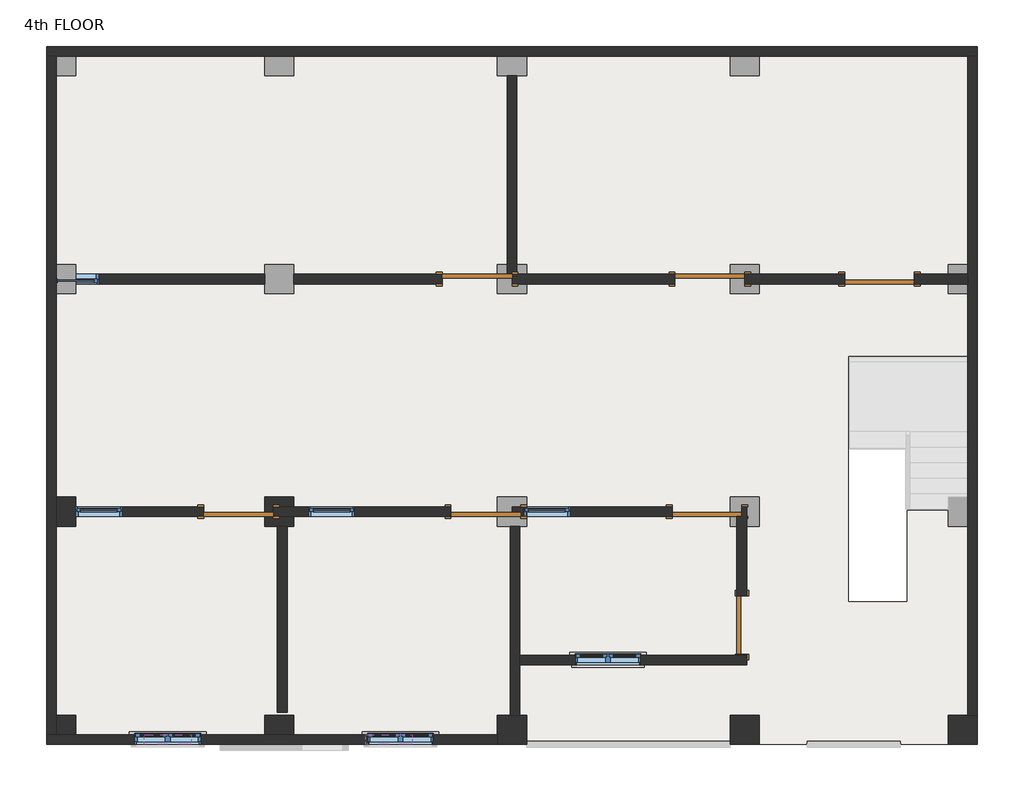
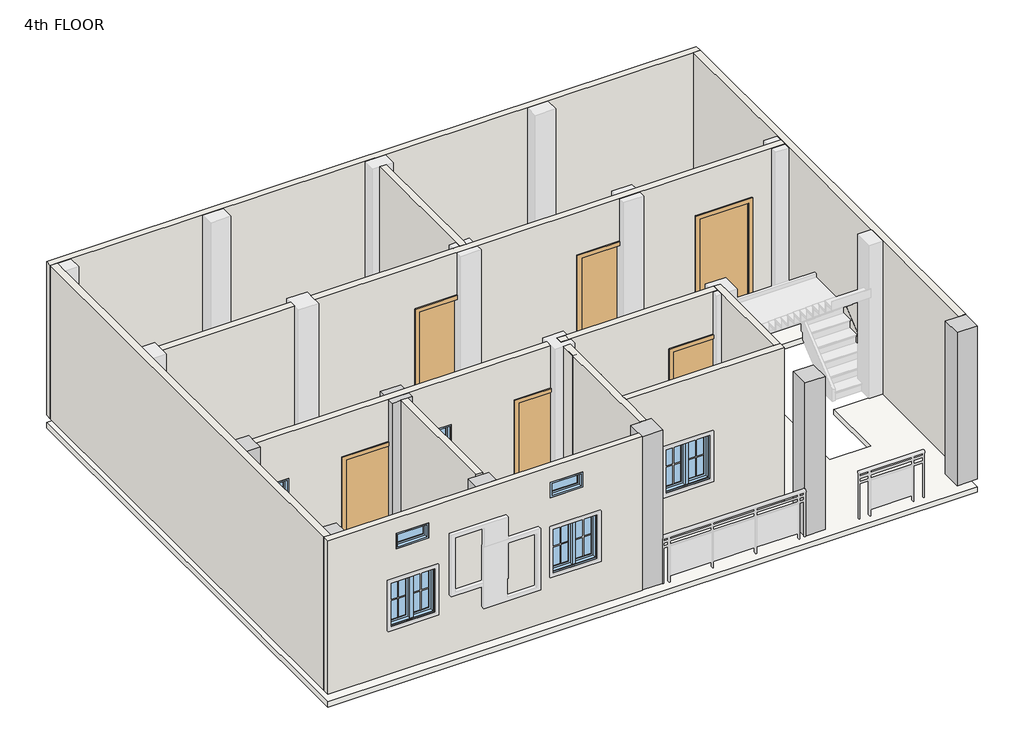
# One storey, part 1 of 2: 15 walls, 9 windows, 7 columns, 7 doors, 1 slab.
"""IFC4 building model written with IfcOpenShell, lengths in millimetres."""

from ifc_helpers import new_model, si_unit, frame, origin, place, context, project, spatial, polyline, outline, extrude, faceted_brep, transform, mapped, element, save
from components import door_e00f436c, door_a1797ceb, window_4c2727af, window_0bf3737e, window_78893e6c, window_0d9958e7

model = new_model("IFC4")

# Units and contexts
model_context = context("Model", 3, world=origin())
ifc_project = project(units=[si_unit("LENGTHUNIT", "METRE", prefix="MILLI")], contexts=[model_context])

# Site, building, storey
site = spatial("IfcSite", under=ifc_project)
building = spatial("IfcBuilding", under=site)
storey = spatial("IfcBuildingStorey", under=building, Name="4th FLOOR", Elevation=12039.6)

# Columns
placement = place(None, origin())
element("IfcColumn", 1, ObjectType="column family : column family", at=placement, inside=storey, context=model_context, shape_type="Brep", body=[
    faceted_brep([(-12576.097125, 2486.2065522, 12044.6), (-12957.097125, 2486.2065522, 12044.6), (-12957.097125, 2867.2065522, 12044.6), (-12576.097125, 2867.2065522, 12044.6), (-12576.097125, 2740.2065522, 12044.6), (-12842.797125, 2740.2065522, 12044.6), (-12842.797125, 2613.2065522, 12044.6), (-12576.097125, 2613.2065522, 12044.6), (-12576.097125, 2486.2065522, 15082.6), (-12576.097125, 2613.2065522, 15082.6), (-12957.097125, 2486.2065522, 15082.6), (-12957.097125, 2613.2065522, 15082.6), (-12957.097125, 2613.2065522, 14173.2), (-12957.097125, 2740.2065522, 14173.2), (-12957.097125, 2740.2065522, 15082.6), (-12957.097125, 2867.2065522, 15082.6), (-12576.097125, 2867.2065522, 15082.6), (-12842.797125, 2613.2065522, 14173.2), (-12842.797125, 2740.2065522, 14173.2), (-12576.097125, 2740.2065522, 15082.6)], [[[0, 1, 2, 3, 4, 5, 6, 7]], [[8, 0, 7, 9]], [[1, 0, 8, 10]], [[2, 1, 10, 11, 12, 13, 14, 15]], [[3, 2, 15, 16]], [[10, 8, 9, 11]], [[6, 17, 12, 11, 9, 7]], [[13, 18, 5, 4, 19, 14]], [[3, 16, 19, 4]], [[16, 15, 14, 19]], [[17, 18, 13, 12]], [[18, 17, 6, 5]]]),
])
element("IfcColumn", 2, ObjectType="column family : column family", at=placement, inside=storey, context=model_context, shape_type="SweptSolid", body=[
    extrude(outline(polyline([(-15433.597125, 2867.2065522), (-15433.597125, 2486.2065522), (-15687.597125, 2486.2065522), (-15687.597125, 2867.2065522), (-15433.597125, 2867.2065522)])), frame((0.0, 0.0, 12044.6), z_axis=(0.0, 0.0, 1.0), x_axis=(1.0, 0.0, 0.0)), (0.0, 0.0, 1.0), 3038.0),
])
element("IfcColumn", 3, ObjectType="column family : column family", at=placement, inside=storey, context=model_context, shape_type="SweptSolid", body=[
    extrude(outline(polyline([(-15433.597125, 9.7065522), (-15433.597125, -244.2934478), (-15687.597125, -244.2934478), (-15687.597125, 9.7065522), (-15433.597125, 9.7065522)])), frame((0.0, 0.0, 12044.6), z_axis=(0.0, 0.0, 1.0), x_axis=(1.0, 0.0, 0.0)), (0.0, 0.0, 1.0), 3038.0),
])
element("IfcColumn", 4, ObjectType="column family : column family", at=placement, inside=storey, context=model_context, shape_type="SweptSolid", body=[
    extrude(outline(polyline([(-3622.597125, 9.7065522), (-3622.597125, -371.2934478), (-4003.597125, -371.2934478), (-4003.597125, 9.7065522), (-3622.597125, 9.7065522)])), frame((0.0, 0.0, 12044.6), z_axis=(0.0, 0.0, 1.0), x_axis=(1.0, 0.0, 0.0)), (0.0, 0.0, 1.0), 3038.0),
])
element("IfcColumn", 5, ObjectType="column family : column family", at=placement, inside=storey, context=model_context, shape_type="SweptSolid", body=[
    extrude(outline(polyline([(-6480.097125, 9.7065522), (-6480.097125, -371.2934478), (-6861.097125, -371.2934478), (-6861.097125, 9.7065522), (-6480.097125, 9.7065522)])), frame((0.0, 0.0, 12044.6), z_axis=(0.0, 0.0, 1.0), x_axis=(1.0, 0.0, 0.0)), (0.0, 0.0, 1.0), 3038.0),
])
element("IfcColumn", 6, ObjectType="column family : column family", at=placement, inside=storey, context=model_context, shape_type="SweptSolid", body=[
    extrude(outline(polyline([(-9528.097125, 9.7065522), (-9528.097125, -371.2934478), (-9909.097125, -371.2934478), (-9909.097125, 9.7065522), (-9528.097125, 9.7065522)])), frame((0.0, 0.0, 12044.6), z_axis=(0.0, 0.0, 1.0), x_axis=(1.0, 0.0, 0.0)), (0.0, 0.0, 1.0), 3038.0),
])
element("IfcColumn", 7, ObjectType="column family : column family", at=placement, inside=storey, context=model_context, shape_type="SweptSolid", body=[
    extrude(outline(polyline([(-12957.097125, 9.7065522), (-12576.097125, 9.7065522), (-12576.097125, -244.2934478), (-12957.097125, -244.2934478), (-12957.097125, 9.7065522)])), frame((0.0, 0.0, 12044.6), z_axis=(0.0, 0.0, 1.0), x_axis=(1.0, 0.0, 0.0)), (0.0, 0.0, 1.0), 3038.0),
])

# Doors
door_shape = door_e00f436c(model_context)
element("IfcDoor", 8, ObjectType="Single-Flush : 30\" x 80\"", at=placement, inside=storey, context=model_context, shape_type="MappedRepresentation", body=[
    mapped(door_shape, transform((-6708.697125, 1190.8065522, 12039.6), x_axis=(0.0, -1.0, 0.0), y_axis=(1.0, 0.0, 0.0), z_axis=(0.0, 0.0, 1.0))),
])
door_2_shape = door_a1797ceb(model_context)
element("IfcDoor", 9, ObjectType="Single-Flush : 36\" x 84\"", at=placement, inside=storey, context=model_context, shape_type="MappedRepresentation", body=[
    mapped(door_2_shape, transform((-10175.797125, 5724.7065522, 12039.6), x_axis=(1.0, 0.0, 0.0), y_axis=(0.0, 1.0, 0.0), z_axis=(0.0, 0.0, 1.0))),
])
element("IfcDoor", 10, ObjectType="Single-Flush : 36\" x 84\"", at=placement, inside=storey, context=model_context, shape_type="MappedRepresentation", body=[
    mapped(door_2_shape, transform((-10061.497125, 2676.7065522, 12039.6), x_axis=(-1.0, 0.0, 0.0), y_axis=(0.0, -1.0, 0.0), z_axis=(0.0, 0.0, 1.0))),
])
element("IfcDoor", 11, ObjectType="Single-Flush : 36\" x 84\"", at=placement, inside=storey, context=model_context, shape_type="MappedRepresentation", body=[
    mapped(door_2_shape, transform((-13299.997125, 2676.7065522, 12039.6), x_axis=(-1.0, 0.0, 0.0), y_axis=(0.0, -1.0, 0.0), z_axis=(0.0, 0.0, 1.0))),
])
element("IfcDoor", 12, ObjectType="Single-Flush : 36\" x 84\"", at=placement, inside=storey, context=model_context, shape_type="MappedRepresentation", body=[
    mapped(door_2_shape, transform((-7127.797125, 5724.7065522, 12039.6), x_axis=(1.0, 0.0, 0.0), y_axis=(0.0, 1.0, 0.0), z_axis=(0.0, 0.0, 1.0))),
])
element("IfcDoor", 13, ObjectType="Single-Flush : 36\" x 84\"", at=placement, inside=storey, context=model_context, shape_type="MappedRepresentation", body=[
    mapped(door_2_shape, transform((-7165.897125, 2676.7065522, 12039.6), x_axis=(-1.0, 0.0, 0.0), y_axis=(0.0, -1.0, 0.0), z_axis=(0.0, 0.0, 1.0))),
])
element("IfcDoor", 14, ObjectType="Single-Flush : 36\" x 84\"", at=placement, inside=storey, context=model_context, shape_type="MappedRepresentation", body=[
    mapped(door_2_shape, transform((-4905.297125, 5724.7065522, 12039.6), x_axis=(-1.0, 0.0, 0.0), y_axis=(0.0, -1.0, 0.0), z_axis=(0.0, 0.0, 1.0))),
])

# Slab
element("IfcSlab", 15, ObjectType="Generic - 4\"", at=placement, inside=storey, context=model_context, shape_type="SweptSolid", body=[
    extrude(outline(polyline([(-3622.597125, 8772.7065522), (-3622.597125, -371.2934478), (-15814.597125, -371.2934478), (-15814.597125, 8772.7065522), (-3622.597125, 8772.7065522)]), holes=[polyline([(-3734.357125, 4711.0719226), (-5310.2646464, 4711.0719226), (-5310.2646464, 1502.3126957), (-4547.7736682, 1502.3126957), (-4547.7736682, 2699.911213), (-3734.357125, 2699.911213), (-3734.357125, 4711.0719226)])]), frame((0.0, 0.0, 11785.6), z_axis=(0.0, 0.0, 1.0), x_axis=(1.0, 0.0, 0.0)), (0.0, 0.0, 1.0), 101.6),
])

# Walls
element("IfcWall", 16, ObjectType="Generic - 5\"", at=placement, inside=storey, context=model_context, shape_type="Brep", body=[
    faceted_brep([(-15814.597125, 8645.7065522, 12039.6), (-15687.597125, 8645.7065522, 12039.6), (-3749.597125, 8645.7065522, 12039.6), (-3622.597125, 8645.7065522, 12039.6), (-3622.597125, 8645.7065522, 15087.6), (-3749.597125, 8645.7065522, 15087.6), (-15687.597125, 8645.7065522, 15087.6), (-15814.597125, 8645.7065522, 15087.6), (-15814.597125, 8772.7065522, 12039.6), (-15814.597125, 8772.7065522, 15087.6), (-3622.597125, 8772.7065522, 15087.6), (-3622.597125, 8772.7065522, 12039.6)], [[[0, 1, 2, 3, 4, 5, 6, 7]], [[8, 9, 10, 11]], [[3, 2, 1, 0, 8, 11]], [[7, 6, 5, 4, 10, 9]], [[4, 3, 11, 10]], [[0, 7, 9, 8]]]),
])
element("IfcWall", 17, ObjectType="Generic - 5\"", at=placement, inside=storey, context=model_context, shape_type="Brep", body=[
    faceted_brep([(-3749.597125, 8645.7065522, 12039.6), (-3749.597125, 5788.2065522, 12039.6), (-3749.597125, 5661.2065522, 12039.6), (-3749.597125, 9.7065522, 12039.6), (-3749.597125, 9.7065522, 15087.6), (-3749.597125, 5661.2065522, 15087.6), (-3749.597125, 5788.2065522, 15087.6), (-3749.597125, 8645.7065522, 15087.6), (-3622.597125, 8645.7065522, 12039.6), (-3622.597125, 8645.7065522, 15087.6), (-3622.597125, 9.7065522, 15087.6), (-3622.597125, 9.7065522, 15082.6), (-3622.597125, 9.7065522, 12044.6), (-3622.597125, 9.7065522, 12039.6)], [[[0, 1, 2, 3, 4, 5, 6, 7]], [[8, 9, 10, 11, 12, 13]], [[3, 2, 1, 0, 8, 13]], [[4, 3, 13, 12, 11, 10]], [[7, 6, 5, 4, 10, 9]], [[0, 7, 9, 8]]]),
])
element("IfcWall", 18, ObjectType="Generic - 5\"", at=placement, inside=storey, context=model_context, shape_type="Brep", body=[
    faceted_brep([(-9909.097125, -244.2934478, 12039.6), (-15687.597125, -244.2934478, 12039.6), (-15814.597125, -244.2934478, 12039.6), (-15814.597125, -244.2934478, 15087.6), (-15687.597125, -244.2934478, 15087.6), (-9909.097125, -244.2934478, 15087.6), (-13795.297125, -244.2934478, 13868.4), (-14658.897125, -244.2934478, 13868.4), (-14658.897125, -244.2934478, 12954.0), (-13795.297125, -244.2934478, 12954.0), (-10747.297125, -244.2934478, 13868.4), (-11610.897125, -244.2934478, 13868.4), (-11610.897125, -244.2934478, 12954.0), (-10747.297125, -244.2934478, 12954.0), (-13922.297125, -244.2934478, 14782.8), (-14531.897125, -244.2934478, 14782.8), (-14531.897125, -244.2934478, 14478.0), (-13922.297125, -244.2934478, 14478.0), (-11026.697125, -244.2934478, 14782.8), (-11636.297125, -244.2934478, 14782.8), (-11636.297125, -244.2934478, 14478.0), (-11026.697125, -244.2934478, 14478.0), (-9909.097125, -371.2934478, 12039.6), (-9909.097125, -371.2934478, 12044.6), (-9909.097125, -371.2934478, 15082.6), (-9909.097125, -371.2934478, 15087.6), (-15814.597125, -371.2934478, 15087.6), (-15814.597125, -371.2934478, 12039.6), (-13795.297125, -371.2934478, 13868.4), (-13795.297125, -371.2934478, 12954.0), (-14658.897125, -371.2934478, 12954.0), (-14658.897125, -371.2934478, 13868.4), (-10747.297125, -371.2934478, 13868.4), (-10747.297125, -371.2934478, 12954.0), (-11610.897125, -371.2934478, 12954.0), (-11610.897125, -371.2934478, 13868.4), (-13922.297125, -371.2934478, 14782.8), (-13922.297125, -371.2934478, 14478.0), (-14531.897125, -371.2934478, 14478.0), (-14531.897125, -371.2934478, 14782.8), (-11026.697125, -371.2934478, 14782.8), (-11026.697125, -371.2934478, 14478.0), (-11636.297125, -371.2934478, 14478.0), (-11636.297125, -371.2934478, 14782.8)], [[[0, 1, 2, 3, 4, 5], [6, 7, 8, 9], [10, 11, 12, 13], [14, 15, 16, 17], [18, 19, 20, 21]], [[22, 23, 24, 25, 26, 27], [28, 29, 30, 31], [32, 33, 34, 35], [36, 37, 38, 39], [40, 41, 42, 43]], [[2, 1, 0, 22, 27]], [[5, 4, 3, 26, 25]], [[0, 5, 25, 24, 23, 22]], [[3, 2, 27, 26]], [[29, 28, 6, 9]], [[30, 29, 9, 8]], [[31, 30, 8, 7]], [[28, 31, 7, 6]], [[33, 32, 10, 13]], [[34, 33, 13, 12]], [[35, 34, 12, 11]], [[32, 35, 11, 10]], [[37, 36, 14, 17]], [[38, 37, 17, 16]], [[39, 38, 16, 15]], [[36, 39, 15, 14]], [[41, 40, 18, 21]], [[42, 41, 21, 20]], [[43, 42, 20, 19]], [[40, 43, 19, 18]]]),
])
element("IfcWall", 19, ObjectType="Generic - 5\"", at=placement, inside=storey, context=model_context, shape_type="Brep", body=[
    faceted_brep([(-15687.597125, -244.2934478, 12039.6), (-15687.597125, 8645.7065522, 12039.6), (-15687.597125, 8645.7065522, 12044.6), (-15687.597125, 8645.7065522, 15082.6), (-15687.597125, 8645.7065522, 15087.6), (-15687.597125, -244.2934478, 15087.6), (-15687.597125, -244.2934478, 15082.6), (-15687.597125, -244.2934478, 12044.6), (-15814.597125, -244.2934478, 12039.6), (-15814.597125, -244.2934478, 15087.6), (-15814.597125, 8645.7065522, 15087.6), (-15814.597125, 8645.7065522, 12039.6)], [[[0, 1, 2, 3, 4, 5, 6, 7]], [[8, 9, 10, 11]], [[1, 0, 8, 11]], [[5, 4, 10, 9]], [[4, 3, 2, 1, 11, 10]], [[0, 7, 6, 5, 9, 8]]]),
])
element("IfcWall", 20, ObjectType="Generic - 5\"", at=placement, inside=storey, context=model_context, shape_type="SweptSolid", body=[
    extrude(outline(polyline([(12039.6, -15433.597125), (12039.6, -12957.097125), (15087.6, -12957.097125), (15087.6, -15433.597125), (14173.2, -15433.597125), (14173.2, -15128.797125), (12344.4, -15128.797125), (12344.4, -15433.597125), (12039.6, -15433.597125)])), frame((0.0, 5661.2065522, 0.0), z_axis=(0.0, 1.0, 0.0), x_axis=(0.0, 0.0, 1.0)), (0.0, 0.0, 1.0), 127.0),
])
element("IfcWall", 21, ObjectType="Generic - 5\"", at=placement, inside=storey, context=model_context, shape_type="Brep", body=[
    faceted_brep([(-9782.097125, 8391.7065522, 12039.6), (-9782.097125, 5788.2065522, 12039.6), (-9782.097125, 5788.2065522, 12044.6), (-9782.097125, 5788.2065522, 14173.2), (-9782.097125, 5788.2065522, 15082.6), (-9782.097125, 5788.2065522, 15087.6), (-9782.097125, 8391.7065522, 15087.6), (-9655.097125, 8391.7065522, 12039.6), (-9655.097125, 8391.7065522, 15087.6), (-9655.097125, 5788.2065522, 15087.6), (-9655.097125, 5788.2065522, 15082.6), (-9655.097125, 5788.2065522, 12044.6), (-9655.097125, 5788.2065522, 12039.6), (-9718.597125, 5788.2065522, 12039.6)], [[[0, 1, 2, 3, 4, 5, 6]], [[7, 8, 9, 10, 11, 12]], [[1, 0, 7, 12, 13]], [[6, 5, 9, 8]], [[0, 6, 8, 7]], [[5, 4, 3, 2, 1, 13, 12, 11, 10, 9]]]),
])
element("IfcWall", 22, ObjectType="Generic - 5\"", at=placement, inside=storey, context=model_context, shape_type="Brep", body=[
    faceted_brep([(-6670.597125, 5661.2065522, 12039.6), (-5362.497125, 5661.2065522, 12039.6), (-5362.497125, 5661.2065522, 14173.2), (-4448.097125, 5661.2065522, 14173.2), (-4448.097125, 5661.2065522, 12039.6), (-3749.597125, 5661.2065522, 12039.6), (-3749.597125, 5661.2065522, 12044.6), (-3749.597125, 5661.2065522, 15082.6), (-3749.597125, 5661.2065522, 15087.6), (-12576.097125, 5661.2065522, 15087.6), (-12576.097125, 5661.2065522, 12039.6), (-10632.997125, 5661.2065522, 12039.6), (-10632.997125, 5661.2065522, 14173.2), (-9909.097125, 5661.2065522, 14173.2), (-9718.597125, 5661.2065522, 14173.2), (-9718.597125, 5661.2065522, 12044.6), (-9718.597125, 5661.2065522, 12039.6), (-7584.997125, 5661.2065522, 12039.6), (-7584.997125, 5661.2065522, 14173.2), (-6861.097125, 5661.2065522, 14173.2), (-6670.597125, 5661.2065522, 14173.2), (-6670.597125, 5661.2065522, 12044.6), (-5362.497125, 5788.2065522, 14173.2), (-5362.497125, 5788.2065522, 12039.6), (-6670.597125, 5788.2065522, 12039.6), (-6670.597125, 5788.2065522, 12044.6), (-6670.597125, 5788.2065522, 14173.2), (-6861.097125, 5788.2065522, 14173.2), (-7584.997125, 5788.2065522, 14173.2), (-7584.997125, 5788.2065522, 12039.6), (-9655.097125, 5788.2065522, 12039.6), (-9718.597125, 5788.2065522, 12039.6), (-9718.597125, 5788.2065522, 12044.6), (-9718.597125, 5788.2065522, 14173.2), (-9782.097125, 5788.2065522, 14173.2), (-9909.097125, 5788.2065522, 14173.2), (-10632.997125, 5788.2065522, 14173.2), (-10632.997125, 5788.2065522, 12039.6), (-12576.097125, 5788.2065522, 12039.6), (-12576.097125, 5788.2065522, 15087.6), (-9782.097125, 5788.2065522, 15087.6), (-9655.097125, 5788.2065522, 15087.6), (-3749.597125, 5788.2065522, 15087.6), (-3749.597125, 5788.2065522, 15082.6), (-3749.597125, 5788.2065522, 12044.6), (-3749.597125, 5788.2065522, 12039.6), (-4448.097125, 5788.2065522, 12039.6), (-4448.097125, 5788.2065522, 14173.2)], [[[0, 1, 2, 3, 4, 5, 6, 7, 8, 9, 10, 11, 12, 13, 14, 15, 16, 17, 18, 19, 20, 21]], [[22, 23, 24, 25, 26, 27, 28, 29, 30, 31, 32, 33, 34, 35, 36, 37, 38, 39, 40, 41, 42, 43, 44, 45, 46, 47]], [[11, 10, 38, 37]], [[17, 16, 31, 30, 29]], [[46, 45, 5, 4]], [[24, 23, 1, 0]], [[9, 8, 42, 41, 40, 39]], [[10, 9, 39, 38]], [[8, 7, 6, 5, 45, 44, 43, 42]], [[33, 32, 31, 16, 15, 14]], [[36, 35, 34, 33, 14, 13, 12]], [[37, 36, 12, 11]], [[26, 25, 24, 0, 21, 20]], [[28, 27, 26, 20, 19, 18]], [[29, 28, 18, 17]], [[2, 1, 23, 22]], [[3, 2, 22, 47]], [[4, 3, 47, 46]]]),
])
element("IfcWall", 23, ObjectType="Generic - 5\"", at=placement, inside=storey, context=model_context, shape_type="Brep", body=[
    faceted_brep([(-14823.997125, 2613.2065522, 12344.4), (-15433.597125, 2613.2065522, 12344.4), (-15433.597125, 2613.2065522, 12039.6), (-13757.197125, 2613.2065522, 12039.6), (-13757.197125, 2613.2065522, 14173.2), (-12957.097125, 2613.2065522, 14173.2), (-12842.797125, 2613.2065522, 14173.2), (-12842.797125, 2613.2065522, 12044.6), (-12842.797125, 2613.2065522, 12039.6), (-10518.697125, 2613.2065522, 12039.6), (-10518.697125, 2613.2065522, 14173.2), (-9909.097125, 2613.2065522, 14173.2), (-9909.097125, 2613.2065522, 15087.6), (-15433.597125, 2613.2065522, 15087.6), (-15433.597125, 2613.2065522, 14173.2), (-14823.997125, 2613.2065522, 14173.2), (-12385.597125, 2613.2065522, 14173.2), (-11775.997125, 2613.2065522, 14173.2), (-11775.997125, 2613.2065522, 12344.4), (-12385.597125, 2613.2065522, 12344.4), (-15433.597125, 2740.2065522, 12039.6), (-15433.597125, 2740.2065522, 12344.4), (-14823.997125, 2740.2065522, 12344.4), (-14823.997125, 2740.2065522, 14173.2), (-15433.597125, 2740.2065522, 14173.2), (-15433.597125, 2740.2065522, 15087.6), (-9909.097125, 2740.2065522, 15087.6), (-9909.097125, 2740.2065522, 14173.2), (-10518.697125, 2740.2065522, 14173.2), (-10518.697125, 2740.2065522, 12039.6), (-12842.797125, 2740.2065522, 12039.6), (-12842.797125, 2740.2065522, 12044.6), (-12842.797125, 2740.2065522, 14173.2), (-12957.097125, 2740.2065522, 14173.2), (-13757.197125, 2740.2065522, 14173.2), (-13757.197125, 2740.2065522, 12039.6), (-12385.597125, 2740.2065522, 14173.2), (-12385.597125, 2740.2065522, 12344.4), (-11775.997125, 2740.2065522, 12344.4), (-11775.997125, 2740.2065522, 14173.2)], [[[0, 1, 2, 3, 4, 5, 6, 7, 8, 9, 10, 11, 12, 13, 14, 15], [16, 17, 18, 19]], [[20, 21, 22, 23, 24, 25, 26, 27, 28, 29, 30, 31, 32, 33, 34, 35], [36, 37, 38, 39]], [[30, 29, 9, 8]], [[20, 35, 3, 2]], [[26, 12, 11, 27]], [[13, 12, 26, 25]], [[14, 13, 25, 24]], [[2, 1, 21, 20]], [[28, 10, 9, 29]], [[10, 28, 27, 11]], [[4, 3, 35, 34]], [[6, 5, 4, 34, 33, 32]], [[8, 7, 6, 32, 31, 30]], [[22, 21, 1, 0]], [[23, 22, 0, 15]], [[24, 23, 15, 14]], [[37, 36, 16, 19]], [[38, 37, 19, 18]], [[39, 38, 18, 17]], [[36, 39, 17, 16]]]),
])
element("IfcWall", 24, ObjectType="Generic - 5\"", at=placement, inside=storey, context=model_context, shape_type="Brep", body=[
    faceted_brep([(-9616.997125, 9.7065522, 12039.6), (-9616.997125, 670.1065522, 12039.6), (-9616.997125, 797.1065522, 12039.6), (-9616.997125, 2486.2065522, 12039.6), (-9616.997125, 2486.2065522, 15087.6), (-9616.997125, 797.1065522, 15087.6), (-9616.997125, 670.1065522, 15087.6), (-9616.997125, 9.7065522, 15087.6), (-9743.997125, 9.7065522, 12039.6), (-9743.997125, 9.7065522, 15087.6), (-9743.997125, 2486.2065522, 15087.6), (-9743.997125, 2486.2065522, 12039.6)], [[[0, 1, 2, 3, 4, 5, 6, 7]], [[8, 9, 10, 11]], [[3, 2, 1, 0, 8, 11]], [[4, 3, 11, 10]], [[7, 6, 5, 4, 10, 9]], [[0, 7, 9, 8]]]),
])
element("IfcWall", 25, ObjectType="Generic - 5\"", at=placement, inside=storey, context=model_context, shape_type="SweptSolid", body=[
    extrude(outline(polyline([(-9743.997125, 2181.4065522), (-9743.997125, 2486.2065522), (-9616.997125, 2486.2065522), (-9616.997125, 2181.4065522), (-9743.997125, 2181.4065522)])), frame((0.0, 0.0, 12039.6), z_axis=(0.0, 0.0, 1.0), x_axis=(1.0, 0.0, 0.0)), (0.0, 0.0, 1.0), 3048.0),
])
element("IfcWall", 26, ObjectType="Generic - 5\"", at=placement, inside=storey, context=model_context, shape_type="Brep", body=[
    faceted_brep([(-6772.197125, 2613.2065522, 15087.6), (-9718.597125, 2613.2065522, 15087.6), (-9718.597125, 2613.2065522, 15082.6), (-9718.597125, 2613.2065522, 12044.6), (-9718.597125, 2613.2065522, 12039.6), (-7623.097125, 2613.2065522, 12039.6), (-7623.097125, 2613.2065522, 14173.2), (-6861.097125, 2613.2065522, 14173.2), (-6772.197125, 2613.2065522, 14173.2), (-6772.197125, 2613.2065522, 15082.6), (-9566.197125, 2613.2065522, 14173.2), (-9528.097125, 2613.2065522, 14173.2), (-8956.597125, 2613.2065522, 14173.2), (-8956.597125, 2613.2065522, 12344.4), (-9528.097125, 2613.2065522, 12344.4), (-9566.197125, 2613.2065522, 12344.4), (-9718.597125, 2740.2065522, 15087.6), (-6772.197125, 2740.2065522, 15087.6), (-6772.197125, 2740.2065522, 14173.2), (-6861.097125, 2740.2065522, 14173.2), (-7623.097125, 2740.2065522, 14173.2), (-7623.097125, 2740.2065522, 12039.6), (-9718.597125, 2740.2065522, 12039.6), (-9718.597125, 2740.2065522, 12044.6), (-9718.597125, 2740.2065522, 15082.6), (-9566.197125, 2740.2065522, 14173.2), (-9566.197125, 2740.2065522, 12344.4), (-9528.097125, 2740.2065522, 12344.4), (-8956.597125, 2740.2065522, 12344.4), (-8956.597125, 2740.2065522, 14173.2), (-9528.097125, 2740.2065522, 14173.2)], [[[0, 1, 2, 3, 4, 5, 6, 7, 8, 9], [10, 11, 12, 13, 14, 15]], [[16, 17, 18, 19, 20, 21, 22, 23, 24], [25, 26, 27, 28, 29, 30]], [[4, 22, 21, 5]], [[1, 0, 17, 16]], [[4, 3, 2, 1, 16, 24, 23, 22]], [[26, 25, 10, 15]], [[28, 27, 26, 15, 14, 13]], [[29, 28, 13, 12]], [[25, 30, 29, 12, 11, 10]], [[20, 6, 5, 21]], [[6, 20, 19, 18, 8, 7]], [[17, 0, 9, 8, 18]]]),
])
element("IfcWall", 27, ObjectType="Generic - 5\"", at=placement, inside=storey, context=model_context, shape_type="Brep", body=[
    faceted_brep([(-6645.197125, 797.1065522, 12039.6), (-6645.197125, 809.8065522, 12039.6), (-6645.197125, 809.8065522, 14071.6), (-6645.197125, 1571.8065522, 14071.6), (-6645.197125, 1571.8065522, 12039.6), (-6645.197125, 2740.2065522, 12039.6), (-6645.197125, 2740.2065522, 12044.6), (-6645.197125, 2740.2065522, 15082.6), (-6645.197125, 2740.2065522, 15087.6), (-6645.197125, 797.1065522, 15087.6), (-6772.197125, 809.8065522, 14071.6), (-6772.197125, 809.8065522, 12039.6), (-6772.197125, 797.1065522, 12039.6), (-6772.197125, 797.1065522, 15087.6), (-6772.197125, 2613.2065522, 15087.6), (-6772.197125, 2740.2065522, 15087.6), (-6772.197125, 2740.2065522, 14173.2), (-6772.197125, 2613.2065522, 14173.2), (-6772.197125, 2613.2065522, 12044.6), (-6772.197125, 2613.2065522, 12039.6), (-6772.197125, 1571.8065522, 12039.6), (-6772.197125, 1571.8065522, 14071.6), (-6708.697125, 2613.2065522, 12039.6), (-6708.697125, 2740.2065522, 12039.6), (-6708.697125, 2613.2065522, 14173.2), (-6708.697125, 2613.2065522, 12044.6), (-6708.697125, 2740.2065522, 14173.2), (-6708.697125, 2740.2065522, 12044.6)], [[[0, 1, 2, 3, 4, 5, 6, 7, 8, 9]], [[10, 11, 12, 13, 14, 15, 16, 17, 18, 19, 20, 21]], [[20, 19, 22, 23, 5, 4]], [[12, 11, 1, 0]], [[9, 8, 15, 14, 13]], [[24, 25, 22, 19, 18, 17]], [[26, 24, 17, 16]], [[22, 25, 24, 26, 27, 23]], [[8, 7, 6, 5, 23, 27, 26, 16, 15]], [[0, 9, 13, 12]], [[2, 1, 11, 10]], [[3, 2, 10, 21]], [[4, 3, 21, 20]]]),
])
element("IfcWall", 28, ObjectType="Generic - 5\"", at=placement, inside=storey, context=model_context, shape_type="Brep", body=[
    faceted_brep([(-9718.597125, 2613.2065522, 12039.6), (-9566.197125, 2613.2065522, 12039.6), (-9566.197125, 2613.2065522, 12344.4), (-9566.197125, 2613.2065522, 14173.2), (-9566.197125, 2613.2065522, 15087.6), (-9718.597125, 2613.2065522, 15087.6), (-9718.597125, 2613.2065522, 15082.6), (-9718.597125, 2613.2065522, 12044.6), (-9718.597125, 2740.2065522, 12039.6), (-9718.597125, 2740.2065522, 12044.6), (-9718.597125, 2740.2065522, 15082.6), (-9718.597125, 2740.2065522, 15087.6), (-9566.197125, 2740.2065522, 15087.6), (-9566.197125, 2740.2065522, 14173.2), (-9566.197125, 2740.2065522, 12344.4), (-9566.197125, 2740.2065522, 12039.6)], [[[0, 1, 2, 3, 4, 5, 6, 7]], [[8, 9, 10, 11, 12, 13, 14, 15]], [[1, 0, 8, 15]], [[4, 3, 2, 1, 15, 14, 13, 12]], [[5, 4, 12, 11]], [[0, 7, 6, 5, 11, 10, 9, 8]]]),
])
element("IfcWall", 29, ObjectType="Generic - 5\"", at=placement, inside=storey, context=model_context, shape_type="SweptSolid", body=[
    extrude(outline(polyline([(-12791.997125, 47.8065522), (-12791.997125, 2486.2065522), (-12664.997125, 2486.2065522), (-12664.997125, 47.8065522), (-12791.997125, 47.8065522)])), frame((0.0, 0.0, 12039.6), z_axis=(0.0, 0.0, 1.0), x_axis=(1.0, 0.0, 0.0)), (0.0, 0.0, 1.0), 3048.0),
])
element("IfcWall", 30, ObjectType="Generic - 5\"", at=placement, inside=storey, context=model_context, shape_type="Brep", body=[
    faceted_brep([(-9616.997125, 670.1065522, 12039.6), (-6645.197125, 670.1065522, 12039.6), (-6645.197125, 670.1065522, 15087.6), (-9616.997125, 670.1065522, 15087.6), (-8029.497125, 670.1065522, 13868.4), (-8029.497125, 670.1065522, 12954.0), (-8893.097125, 670.1065522, 12954.0), (-8893.097125, 670.1065522, 13868.4), (-9616.997125, 797.1065522, 12039.6), (-9616.997125, 797.1065522, 15087.6), (-6772.197125, 797.1065522, 15087.6), (-6645.197125, 797.1065522, 15087.6), (-6645.197125, 797.1065522, 12039.6), (-6772.197125, 797.1065522, 12039.6), (-8029.497125, 797.1065522, 13868.4), (-8893.097125, 797.1065522, 13868.4), (-8893.097125, 797.1065522, 12954.0), (-8029.497125, 797.1065522, 12954.0)], [[[0, 1, 2, 3], [4, 5, 6, 7]], [[8, 9, 10, 11, 12, 13], [14, 15, 16, 17]], [[1, 0, 8, 13, 12]], [[3, 2, 11, 10, 9]], [[0, 3, 9, 8]], [[2, 1, 12, 11]], [[5, 4, 14, 17]], [[6, 5, 17, 16]], [[7, 6, 16, 15]], [[4, 7, 15, 14]]]),
])

# Windows
window_shape = window_4c2727af(model_context)
element("IfcWindow", 31, ObjectType="Fixed : 24\" x 12\"", at=placement, inside=storey, context=model_context, shape_type="MappedRepresentation", body=[
    mapped(window_shape, transform((-14188.997125, -307.7934478, 13563.6), x_axis=(1.0, 0.0, 0.0), y_axis=(0.0, 1.0, 0.0), z_axis=(0.0, 0.0, 1.0))),
])
element("IfcWindow", 32, ObjectType="Fixed : 24\" x 12\"", at=placement, inside=storey, context=model_context, shape_type="MappedRepresentation", body=[
    mapped(window_shape, transform((-11293.397125, -307.7934478, 13563.6), x_axis=(1.0, 0.0, 0.0), y_axis=(0.0, 1.0, 0.0), z_axis=(0.0, 0.0, 1.0))),
])
window_2_shape = window_0bf3737e(model_context)
element("IfcWindow", 33, ObjectType="Fixed : 24\" x 72\"", at=placement, inside=storey, context=model_context, shape_type="MappedRepresentation", body=[
    mapped(window_2_shape, transform((-15471.697125, 5724.7065522, 12039.6), x_axis=(-1.0, 0.0, 0.0), y_axis=(0.0, -1.0, 0.0), z_axis=(0.0, 0.0, 1.0))),
])
window_3_shape = window_78893e6c(model_context)
element("IfcWindow", 34, ObjectType="Fixed : 24\" x 72\"", at=placement, inside=storey, context=model_context, shape_type="MappedRepresentation", body=[
    mapped(window_3_shape, transform((-15166.897125, 2676.7065522, 12039.6), x_axis=(-1.0, 0.0, 0.0), y_axis=(0.0, -1.0, 0.0), z_axis=(0.0, 0.0, 1.0))),
])
element("IfcWindow", 35, ObjectType="Fixed : 24\" x 72\"", at=placement, inside=storey, context=model_context, shape_type="MappedRepresentation", body=[
    mapped(window_3_shape, transform((-12118.897125, 2676.7065522, 12039.6), x_axis=(-1.0, 0.0, 0.0), y_axis=(0.0, -1.0, 0.0), z_axis=(0.0, 0.0, 1.0))),
])
element("IfcWindow", 36, ObjectType="Fixed : 24\" x 72\"", at=placement, inside=storey, context=model_context, shape_type="MappedRepresentation", body=[
    mapped(window_3_shape, transform((-9299.497125, 2676.7065522, 12039.6), x_axis=(-1.0, 0.0, 0.0), y_axis=(0.0, -1.0, 0.0), z_axis=(0.0, 0.0, 1.0))),
])
window_4_shape = window_0d9958e7(model_context)
element("IfcWindow", 37, ObjectType="Window-Casement-Double : 34\" x 36\"", at=placement, inside=storey, context=model_context, shape_type="MappedRepresentation", body=[
    mapped(window_4_shape, transform((-14227.097125, -307.7934478, 12039.6), x_axis=(1.0, 0.0, 0.0), y_axis=(0.0, 1.0, 0.0), z_axis=(0.0, 0.0, 1.0))),
])
element("IfcWindow", 38, ObjectType="Window-Casement-Double : 34\" x 36\"", at=placement, inside=storey, context=model_context, shape_type="MappedRepresentation", body=[
    mapped(window_4_shape, transform((-11179.097125, -307.7934478, 12039.6), x_axis=(1.0, 0.0, 0.0), y_axis=(0.0, 1.0, 0.0), z_axis=(0.0, 0.0, 1.0))),
])
element("IfcWindow", 39, ObjectType="Window-Casement-Double : 34\" x 36\"", at=placement, inside=storey, context=model_context, shape_type="MappedRepresentation", body=[
    mapped(window_4_shape, transform((-8461.297125, 733.6065522, 12039.6), x_axis=(1.0, 0.0, 0.0), y_axis=(0.0, 1.0, 0.0), z_axis=(0.0, 0.0, 1.0))),
])

save(model, "model.ifc")

# Revit data of these elements
# Type "column family : column family"
#   w2 [instance default] = 0' - 9.88189"
#   w1 [instance default] = 0' - 9.01575"
#   Depth = 1' - 11.62205"
#   Width = 1' - 11.62205"
# Type "Single-Flush : 30\" x 80\""
#   Type Mark = "5"
#   Construction Type Id = "MDOOR"
#   Assembly Code = "C1020"
#   Analytic Construction = "Metal"
#   Thickness = 0' - 2"
#   Heat Transfer Coefficient (U) = 0.651978 BTU/(h·ft²·°F)
#   Height = 6' - 8"
#   Trim Projection Ext = 0' - 1"
#   Trim Projection Int = 0' - 1"
#   Trim Width = 0' - 3"
#   Width = 2' - 6"
#   Define Thermal Properties by = 1
#   Define Thermal Properties by = 1
#   Door Material = Door - Panel
#   Frame Material = Door - Frame
#   Visual Light Transmittance = 0
#   Solar Heat Gain Coefficient = 0
#   Function = (empty or 0)
#   Wall Closure = (empty or 0)
# Type "Single-Flush : 36\" x 84\""
#   Type Mark = "1"
#   Construction Type Id = "MDOOR"
#   Assembly Code = "C1020"
#   Analytic Construction = "Metal"
#   Thickness = 0' - 2"
#   Heat Transfer Coefficient (U) = 0.651978 BTU/(h·ft²·°F)
#   Height = 7' - 0"
#   Trim Projection Ext = 0' - 1"
#   Trim Projection Int = 0' - 1"
#   Trim Width = 0' - 3"
#   Width = 3' - 0"
#   Define Thermal Properties by = 1
#   Define Thermal Properties by = 1
#   Door Material = Door - Panel
#   Frame Material = Door - Frame
#   Visual Light Transmittance = 0
#   Solar Heat Gain Coefficient = 0
#   Function = (empty or 0)
#   Wall Closure = (empty or 0)
# Type "Generic - 4\""
#   Assembly Code = "B1010"
#   Function = 0
#   Layers, outside or top first: 0' - 4" no material (function 1)
# Type "Generic - 5\""
#   Assembly Code = "B2010"
#   Layers, outside or top first: 0' - 5" no material (function 1)
# Type "Fixed : 24\" x 12\""
#   Type Mark = "4"
#   Construction Type Id = "GSP4R"
#   Assembly Code = "B2020100"
#   Analytic Construction = "1/8 in Pilkington single glazing"
#   Visual Light Transmittance = 0.9
#   Solar Heat Gain Coefficient = 0.78
#   Heat Transfer Coefficient (U) = 0.6496 BTU/(h·ft²·°F)
#   Height = 1' - 0"
#   Default Sill Height = 3' - 0"
#   Width = 2' - 0"
#   Window Inset = 0' - 0 3/4"
#   Define Thermal Properties by = 1
#   Define Thermal Properties by = 1
#   Glass Pane Material = Glass
#   Sash Material = Sash
#   Wall Closure = (empty or 0)
# Type "Fixed : 24\" x 72\""
#   Type Mark = "7"
#   Construction Type Id = "GSP4R"
#   Assembly Code = "B2020100"
#   Analytic Construction = "1/8 in Pilkington single glazing"
#   Visual Light Transmittance = 0.9
#   Solar Heat Gain Coefficient = 0.78
#   Heat Transfer Coefficient (U) = 0.6496 BTU/(h·ft²·°F)
#   Height = 6' - 0"
#   Default Sill Height = 1' - 0"
#   Width = 2' - 0"
#   Window Inset = 0' - 0 3/4"
#   Define Thermal Properties by = 1
#   Define Thermal Properties by = 1
#   Glass Pane Material = Glass
#   Sash Material = Sash
#   Wall Closure = (empty or 0)
# Type "Window-Casement-Double : 34\" x 36\""
#   Type Mark = "14"
#   Fire Rating = "0.5h"
#   Assembly Code = "B2020100"
#   Analytic Construction = "Double glazing - domestic"
#   Frame Extension [instance default] = 0' - 0 1/4"
#   Window Inset [instance default] = 0' - 0"
#   Wall Thickness [instance default] = 0' - 6"
#   Interior Wall Closure [instance default] = 0' - 2 1/4"
#   Half Width = 1' - 5"
#   Visual Light Transmittance = 0.81
#   Thermal Resistance (R) = 1.8146 (h·ft²·°F)/BTU
#   Solar Heat Gain Coefficient = 0.76
#   Rough Width = 2' - 10 1/2"
#   Rough Height = 3' - 0 1/2"
#   Height = 3' - 0"
#   Heat Transfer Coefficient (U) = 0.5511 BTU/(h·ft²·°F)
#   Exterior Wall Closure [instance default] = 0' - 1 1/4"
#   Extension Jamb [instance default] = 0' - 2 1/4"
#   Default Sill Height = 3' - 0"
#   Width = 2' - 10"
#   Define Thermal Properties by = 0
#   Muntin Visibility = yes
#   Interior Trim Visibility [instance default] = yes
#   Exterior Trim Visibility [instance default] = yes
#   Extension Jamb Visibility [instance default] = yes
#   Interior Trim Material = Wood - Stained
#   Muntin Pattern = Muntin Pattern_2x2 : Muntin Pattern_2x2
#   Interior Trim = Trim-Window-Interior-Flat : Picture Frame
#   Interior Frame Material = Wood - Stained
#   Glass Panel Material = Glass
#   Exterior Trim Material = Clad - White
#   Exterior Trim = Trim-Window-Exterior-Flat : with Sill
#   Exterior Frame Material = Clad - White
#   Wall Closure = (empty or 0)
# Element 1 (IfcColumn, "column family : column family")
#   w2 = 1' - 3"
#   w1 = 1' - 3"
#   Phase Created = New Construction
#   Materials on its faces: "Default Wall", "inside wall"
# Element 2 (IfcColumn, "column family : column family")
#   w2 = 1' - 3"
#   w1 = 0' - 10"
#   Phase Created = New Construction
#   Materials on its faces: "inside wall", "Default Wall"
# Elements 3, 7 (IfcColumn, "column family : column family")
#   w2 = 1' - 3"
#   w1 = 1' - 3"
#   Phase Created = New Construction
#   Materials on its faces: "Default Wall"
# Element 4 (IfcColumn, "column family : column family")
#   w2 = 1' - 3"
#   w1 = 1' - 3"
#   Phase Created = New Construction
#   Materials on its faces: "Clad - White", "Default Wall"
# Element 5 (IfcColumn, "column family : column family")
#   w2 = 1' - 3"
#   w1 = 1' - 3"
#   Phase Created = New Construction
#   Materials on its faces: "out side wall"
# Element 6 (IfcColumn, "column family : column family")
#   w2 = 1' - 3"
#   w1 = 1' - 3"
#   Phase Created = New Construction
#   Materials on its faces: "out side wall", "Default Wall"
# Element 8 (IfcDoor, "Single-Flush : 30\" x 80\"")
#   Phase Created = New Construction
#   Materials on its faces: "Door - Frame", "Door - Panel"
# Elements 9, 10, 11, 12, 13, 14 (IfcDoor, "Single-Flush : 36\" x 84\"")
#   Phase Created = New Construction
#   Materials on its faces: "Door - Frame", "Door - Panel"
# Element 15 (IfcSlab, "Generic - 4\"")
#   Height Offset From Level = -0' - 6"
#   Phase Created = New Construction
#   Materials on its faces: "Default Floor", "Clad - White", "floor"
# Element 16 (IfcWall, "Generic - 5\"")
#   Top Offset = 0' - 0"
#   Base Offset = 0' - 0"
#   wall height = 10' - 0"
#   Phase Created = New Construction
#   Base Constraint = 4th FLOOR
#   Top Constraint = 5th FLOOR
#   Materials on its faces: "Default Wall", "Clad - White"
# Element 17 (IfcWall, "Generic - 5\"")
#   Top Offset = 0' - 0"
#   Base Offset = 0' - 0"
#   wall height = 10' - 0"
#   Phase Created = New Construction
#   Base Constraint = 4th FLOOR
#   Top Constraint = 5th FLOOR
#   Materials on its faces: "Default Wall", "grey", "Clad - White"
# Element 18 (IfcWall, "Generic - 5\"")
#   Top Offset = 0' - 0"
#   Base Offset = 0' - 0"
#   wall height = 10' - 0"
#   Phase Created = New Construction
#   Base Constraint = 4th FLOOR
#   Top Constraint = 5th FLOOR
#   Materials on its faces: "Default Wall", "out side wall", "Clad - White"
# Element 19 (IfcWall, "Generic - 5\"")
#   Top Offset = 0' - 0"
#   Base Offset = 0' - 0"
#   wall height = 10' - 0"
#   Phase Created = New Construction
#   Base Constraint = 4th FLOOR
#   Top Constraint = 5th FLOOR
#   Materials on its faces: "Default Wall", "inside wall", "Clad - White"
# Elements 20, 23, 26, 27 (IfcWall, "Generic - 5\"")
#   Top Offset = 0' - 0"
#   Base Offset = 0' - 0"
#   wall height = 10' - 0"
#   Phase Created = New Construction
#   Base Constraint = 4th FLOOR
#   Top Constraint = 5th FLOOR
#   Materials on its faces: "Default Wall", "inside wall"
# Elements 21, 25, 28, 29 (IfcWall, "Generic - 5\"")
#   Top Offset = 0' - 0"
#   Base Offset = 0' - 0"
#   wall height = 10' - 0"
#   Phase Created = New Construction
#   Base Constraint = 4th FLOOR
#   Top Constraint = 5th FLOOR
#   Materials on its faces: "Default Wall"
# Elements 22, 24 (IfcWall, "Generic - 5\"")
#   Top Offset = 0' - 0"
#   Base Offset = 0' - 0"
#   wall height = 10' - 0"
#   Phase Created = New Construction
#   Base Constraint = 4th FLOOR
#   Top Constraint = 5th FLOOR
#   Materials on its faces: "Default Wall", "grey"
# Element 30 (IfcWall, "Generic - 5\"")
#   Top Offset = 0' - 0"
#   Base Offset = 0' - 0"
#   wall height = 10' - 0"
#   Phase Created = New Construction
#   Base Constraint = 4th FLOOR
#   Top Constraint = 5th FLOOR
#   Materials on its faces: "Default Wall", "grey", "inside wall"
# Element 31 (IfcWindow, "Fixed : 24\" x 12\"")
#   Mark = "43"
#   Phase Created = New Construction
#   Materials on its faces: "Sash", "Glass"
# Element 32 (IfcWindow, "Fixed : 24\" x 12\"")
#   Mark = "44"
#   Phase Created = New Construction
#   Materials on its faces: "Sash", "Glass"
# Element 33 (IfcWindow, "Fixed : 24\" x 72\"")
#   Mark = "37"
#   Phase Created = New Construction
#   Materials on its faces: "Sash", "Glass"
# Element 34 (IfcWindow, "Fixed : 24\" x 72\"")
#   Mark = "38"
#   Phase Created = New Construction
#   Materials on its faces: "Sash", "Glass"
# Element 35 (IfcWindow, "Fixed : 24\" x 72\"")
#   Mark = "39"
#   Phase Created = New Construction
#   Materials on its faces: "Sash", "Glass"
# Element 36 (IfcWindow, "Fixed : 24\" x 72\"")
#   Mark = "40"
#   Phase Created = New Construction
#   Materials on its faces: "Sash", "Glass"
# Element 37 (IfcWindow, "Window-Casement-Double : 34\" x 36\"")
#   Mark = "41"
#   Window Inset = 0' - 0"
#   Interior Wall Closure = 0' - 2 1/4"
#   Frame Extension = 0' - 0 1/4"
#   Exterior Wall Closure = 0' - 1 1/4"
#   Interior Trim Visibility = yes
#   Exterior Trim Visibility = yes
#   Phase Created = New Construction
#   Materials on its faces: "Wood - Stained", "Glass", "Clad - White"
# Element 38 (IfcWindow, "Window-Casement-Double : 34\" x 36\"")
#   Mark = "42"
#   Window Inset = 0' - 0"
#   Interior Wall Closure = 0' - 2 1/4"
#   Frame Extension = 0' - 0 1/4"
#   Exterior Wall Closure = 0' - 1 1/4"
#   Interior Trim Visibility = yes
#   Exterior Trim Visibility = yes
#   Phase Created = New Construction
#   Materials on its faces: "Wood - Stained", "Glass", "Clad - White"
# Element 39 (IfcWindow, "Window-Casement-Double : 34\" x 36\"")
#   Mark = "45"
#   Window Inset = 0' - 0"
#   Interior Wall Closure = 0' - 2 1/4"
#   Frame Extension = 0' - 0 1/4"
#   Exterior Wall Closure = 0' - 1 1/4"
#   Interior Trim Visibility = yes
#   Exterior Trim Visibility = yes
#   Phase Created = New Construction
#   Materials on its faces: "Wood - Stained", "Glass", "Clad - White"
# Materials
#   "Door - Panel": class "Wood", colour RGB 210 159 95, transparency 0, Cost = 0
#   "Door - Frame": colour RGB 118 70 51, transparency 0, Cost = 0
#   "Glass": class "Glass", colour RGB 0 128 192, transparency 0.75, Description = "Soda Lime Glass", Cost = 0
#   "Sash": class "Wood", colour RGB 224 178 126, transparency 0, Cost = 0
#   "Wood - Stained": class "Wood", colour RGB 224 178 126, transparency 0, Cost = 0
#   "Clad - White": class "Wood", colour RGB 242 242 238, transparency 0, Cost = 0
#   "Default Wall": colour RGB 128 128 128, transparency 0, Cost = 0
#   "inside wall": class "Generic", colour RGB 199 224 95, transparency 0, Cost = 0
#   "out side wall": class "Generic", colour RGB 16 106 159, transparency 0, Cost = 0
#   "Default Floor": colour RGB 128 128 128, transparency 0, Cost = 0
#   "floor": class "Generic", colour RGB 255 255 255, transparency 0, Cost = 0
#   "grey": class "Generic", colour RGB 80 80 80, transparency 0, Cost = 0
